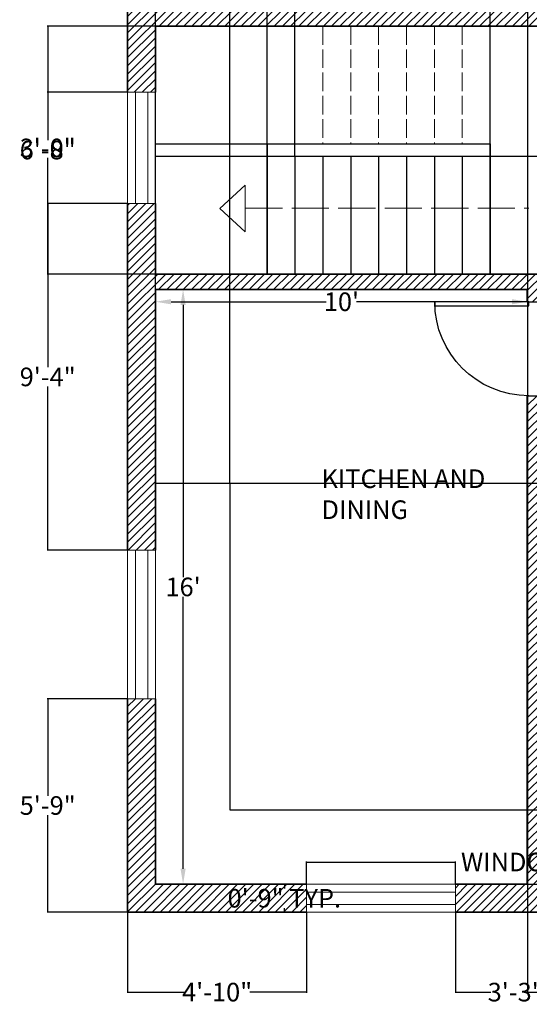
# Model space of a CAD drawing. Units: inches. Extents: x -302 to 383, y -29 to 550.
# Tile 1 of 4: x -17 to 147, y -9 to 308. Entities that reach past the tile are written whole.
import ezdxf

# ---------------------------------------------------------------- set-up
doc = ezdxf.new("R2010")
doc.units = ezdxf.units.IN
doc.header["$MEASUREMENT"] = 0
doc.linetypes.add('ACAD_ISO02W100', pattern=[15, 12, -3])
for name, color, linetype, lineweight in [('A-ANNO-DIMS', 3, 'Continuous', 18), ('A-ANNO-SYMB', 7, 'ACAD_ISO02W100', 18), ('A-AREA-IDEN', 2, 'Continuous', 25), ('A-DOOR', 4, 'Continuous', 25), ('A-FLOR-CASE', 7, 'Continuous', 25), ('A-FLOR-STRS', 7, 'Continuous', 25), ('A-FLOR-STRS-OVHD', 7, 'ACAD_ISO02W100', 18), ('A-GLAZ', 2, 'Continuous', 18), ('A-WALL', 7, 'Continuous', 35), ('A-WALL-PATT', 252, 'Continuous', 13)]:
    doc.layers.add(name, color=color, linetype=linetype, lineweight=lineweight)
doc.styles.get("Standard").update_dxf_attribs({"font": 'arial.ttf'})
doc.dimstyles.get("Standard").update_dxf_attribs({"dimtxt": 6, "dimasz": 0.18, "dimexe": 0.18, "dimexo": 0.0625, "dimgap": 0.09, "dimtad": 0, "dimtih": 1, "dimtoh": 1, "dimzin": 0, "dimdsep": 46, "dimlunit": 3, "dimtxsty": 'Standard', "dimcen": 0.09, "dimadec": 0, "dimazin": 0, "dimtfac": 1, "dimtofl": 0, "dimtmove": 0, "dimatfit": 3, "dimfxl": 1, "dimtolj": 1, "dimtzin": 0, "dimarcsym": 0})

# ---------------------------------------------------------------- blocks, each defined once
blk = doc.blocks.new('*U2')
for p, q in [((0, 0), (0, -6)), ((40, 0), (40, -6))]:
    blk.add_line(p, q)
blk.add_lwpolyline([(0, 0), (0, 40), (1.75, 40), (1.75, 0)], close=True)
blk.add_arc((0, 0), 40, 0, 90)
blk = doc.blocks.new('*D19')
at = {"layer": 'A-ANNO-DIMS', "color": 0, "lineweight": -2, "transparency": 16777216}
for p, q in [((26.76, 221.27), (35.77, 221.27)), ((35.59, 216.27), (35.59, 128.43)), ((35.59, 34.27), (35.59, 122.12)), ((26.76, 29.27), (35.77, 29.27))]:
    blk.add_line(p, q, dxfattribs=at)
at = {"layer": 'A-ANNO-DIMS', "color": 0, "transparency": 16777216}
for points in [[(34.76, 216.27), (36.42, 216.27), (35.59, 221.27)], [(34.76, 34.27), (36.42, 34.27), (35.59, 29.27)]]:
    blk.add_solid(points, dxfattribs=at)
at = {"layer": 'Defpoints', "color": 0, "transparency": 16777216}
for p in [(26.7, 221.27), (26.7, 29.27), (35.59, 29.27)]:
    blk.add_point(p, dxfattribs=at)
at = {"layer": 'A-ANNO-DIMS', "color": 0, "transparency": 16777216, "insert": (35.59, 125.27), "char_height": 6, "attachment_point": 5}
blk.add_mtext("\\A1;16'", dxfattribs=at)
blk = doc.blocks.new('*D20')
at = {"layer": 'A-ANNO-DIMS', "color": 0, "lineweight": -2, "transparency": 16777216}
for p, q in [((26.7, 221.21), (26.7, 217.14)), ((31.7, 217.32), (81.8, 217.32)), ((141.7, 217.32), (91.6, 217.32)), ((146.7, 217.39), (146.7, 217.5))]:
    blk.add_line(p, q, dxfattribs=at)
at = {"layer": 'A-ANNO-DIMS', "color": 0, "transparency": 16777216}
for points in [[(31.7, 218.16), (31.7, 216.49), (26.7, 217.32)], [(141.7, 218.16), (141.7, 216.49), (146.7, 217.32)]]:
    blk.add_solid(points, dxfattribs=at)
at = {"layer": 'Defpoints', "color": 0, "transparency": 16777216}
for p in [(26.7, 221.27), (146.7, 217.32), (146.7, 217.32)]:
    blk.add_point(p, dxfattribs=at)
at = {"layer": 'A-ANNO-DIMS', "color": 0, "transparency": 16777216, "insert": (86.7, 217.32), "char_height": 6, "attachment_point": 5}
blk.add_mtext("\\A1;10'", dxfattribs=at)
blk = doc.blocks.new('WIN-48IN')
blk.add_lwpolyline([(0, 9), (48, 9), (48, 0), (0, 0)], close=True)
for points in [[(0, 6.5), (48, 6.5)], [(0, 2.5), (48, 2.5)]]:
    blk.add_lwpolyline(points)
blk = doc.blocks.new('*D29')
at = {"layer": 'A-ANNO-DIMS', "color": 0, "lineweight": -2, "transparency": 16777216}
for p, q in [((75.47, 29.34), (75.47, 36.65)), ((75.65, 36.47), (123.29, 36.47)), ((123.47, 29.34), (123.47, 36.65)), ((123.47, 36.47), (123.65, 36.47))]:
    blk.add_line(p, q, dxfattribs=at)
at = {"layer": 'A-ANNO-DIMS', "color": 0, "transparency": 16777216}
for points in [[(75.65, 36.5), (75.65, 36.44), (75.47, 36.47)], [(123.29, 36.5), (123.29, 36.44), (123.47, 36.47)]]:
    blk.add_solid(points, dxfattribs=at)
at = {"layer": 'Defpoints', "color": 0, "transparency": 16777216}
for p in [(123.47, 36.47), (75.47, 29.27), (123.47, 29.27)]:
    blk.add_point(p, dxfattribs=at)
at = {"layer": 'A-ANNO-DIMS', "color": 0, "transparency": 16777216, "insert": (161.7, 36.47), "char_height": 6, "attachment_point": 5}
blk.add_mtext('\\A1;WINDOW 4\'-0" TYP.', dxfattribs=at)
blk = doc.blocks.new('*D30')
at = {"layer": 'A-ANNO-DIMS', "color": 0, "lineweight": -2, "transparency": 16777216}
for p, q in [((75.41, 29.27), (68.09, 29.27)), ((68.27, 29.09), (68.27, 27.93)), ((75.41, 20.27), (68.09, 20.27)), ((68.27, 20.45), (68.27, 21.62))]:
    blk.add_line(p, q, dxfattribs=at)
at = {"layer": 'A-ANNO-DIMS', "color": 0, "transparency": 16777216}
for points in [[(68.24, 29.09), (68.3, 29.09), (68.27, 29.27)], [(68.24, 20.45), (68.3, 20.45), (68.27, 20.27)]]:
    blk.add_solid(points, dxfattribs=at)
at = {"layer": 'Defpoints', "color": 0, "transparency": 16777216}
for p in [(68.27, 29.27), (75.47, 29.27), (75.47, 20.27)]:
    blk.add_point(p, dxfattribs=at)
at = {"layer": 'A-ANNO-DIMS', "color": 0, "transparency": 16777216, "insert": (68.27, 24.77), "char_height": 6, "attachment_point": 5}
blk.add_mtext('\\A1;0\'-9" TYP.', dxfattribs=at)
blk = doc.blocks.new('*D37')
at = {"layer": 'A-ANNO-DIMS', "color": 0, "lineweight": -2, "transparency": 16777216}
for p, q in [((17.7, 20.21), (17.7, -5.71)), ((75.47, 20.21), (75.47, -5.71)), ((17.88, -5.53), (36.07, -5.53)), ((75.29, -5.53), (57.1, -5.53))]:
    blk.add_line(p, q, dxfattribs=at)
at = {"layer": 'A-ANNO-DIMS', "color": 0, "transparency": 16777216}
for points in [[(17.88, -5.5), (17.88, -5.56), (17.7, -5.53)], [(75.29, -5.5), (75.29, -5.56), (75.47, -5.53)]]:
    blk.add_solid(points, dxfattribs=at)
at = {"layer": 'Defpoints', "color": 0, "transparency": 16777216}
for p in [(17.7, 20.27), (75.47, 20.27), (75.47, -5.53)]:
    blk.add_point(p, dxfattribs=at)
at = {"layer": 'A-ANNO-DIMS', "color": 0, "transparency": 16777216, "insert": (46.58, -5.53), "char_height": 6, "attachment_point": 5}
blk.add_mtext('\\A1;4\'-10"', dxfattribs=at)
blk = doc.blocks.new('*D38')
at = {"layer": 'A-ANNO-DIMS', "color": 0, "lineweight": -2, "transparency": 16777216}
for p, q in [((123.47, 20.21), (123.47, -5.71)), ((162.44, 20.21), (162.44, -5.71)), ((123.65, -5.53), (134.89, -5.53)), ((162.26, -5.53), (151.02, -5.53))]:
    blk.add_line(p, q, dxfattribs=at)
at = {"layer": 'A-ANNO-DIMS', "color": 0, "transparency": 16777216}
for points in [[(123.65, -5.5), (123.65, -5.56), (123.47, -5.53)], [(162.26, -5.5), (162.26, -5.56), (162.44, -5.53)]]:
    blk.add_solid(points, dxfattribs=at)
at = {"layer": 'Defpoints', "color": 0, "transparency": 16777216}
for p in [(123.47, 20.27), (162.44, 20.27), (162.44, -5.53)]:
    blk.add_point(p, dxfattribs=at)
at = {"layer": 'A-ANNO-DIMS', "color": 0, "transparency": 16777216, "insert": (142.95, -5.53), "char_height": 6, "attachment_point": 5}
blk.add_mtext('\\A1;3\'-3"', dxfattribs=at)
blk = doc.blocks.new('*D41')
at = {"layer": 'A-ANNO-DIMS', "color": 0, "lineweight": -2, "transparency": 16777216}
for p, q in [((17.63, 89.14), (-8.28, 89.14)), ((-8.1, 88.96), (-8.1, 57.86)), ((-8.1, 20.45), (-8.1, 51.55)), ((17.63, 20.27), (-8.28, 20.27))]:
    blk.add_line(p, q, dxfattribs=at)
at = {"layer": 'A-ANNO-DIMS', "color": 0, "transparency": 16777216}
for points in [[(-8.13, 88.96), (-8.07, 88.96), (-8.1, 89.14)], [(-8.13, 20.45), (-8.07, 20.45), (-8.1, 20.27)]]:
    blk.add_solid(points, dxfattribs=at)
at = {"layer": 'Defpoints', "color": 0, "transparency": 16777216}
for p in [(-8.1, 89.14), (17.7, 89.14), (17.7, 20.27)]:
    blk.add_point(p, dxfattribs=at)
at = {"layer": 'A-ANNO-DIMS', "color": 0, "transparency": 16777216, "insert": (-8.1, 54.71), "char_height": 6, "attachment_point": 5}
blk.add_mtext('\\A1;5\'-9"', dxfattribs=at)
blk = doc.blocks.new('*D42')
at = {"layer": 'A-ANNO-DIMS', "color": 0, "lineweight": -2, "transparency": 16777216}
for p, q in [((17.63, 248.98), (-8.28, 248.98)), ((-8.1, 248.8), (-8.1, 196.22)), ((-8.1, 137.32), (-8.1, 189.91)), ((17.63, 137.14), (-8.28, 137.14))]:
    blk.add_line(p, q, dxfattribs=at)
at = {"layer": 'A-ANNO-DIMS', "color": 0, "transparency": 16777216}
for points in [[(-8.13, 248.8), (-8.07, 248.8), (-8.1, 248.98)], [(-8.13, 137.32), (-8.07, 137.32), (-8.1, 137.14)]]:
    blk.add_solid(points, dxfattribs=at)
at = {"layer": 'Defpoints', "color": 0, "transparency": 16777216}
for p in [(-8.1, 248.98), (17.7, 248.98), (17.7, 137.14)]:
    blk.add_point(p, dxfattribs=at)
at = {"layer": 'A-ANNO-DIMS', "color": 0, "transparency": 16777216, "insert": (-8.1, 193.06), "char_height": 6, "attachment_point": 5}
blk.add_mtext('\\A1;9\'-4"', dxfattribs=at)
blk = doc.blocks.new('*D43')
at = {"layer": 'A-ANNO-DIMS', "color": 0, "lineweight": -2, "transparency": 16777216}
for p, q in [((17.63, 284.93), (-8.28, 284.93)), ((-8.1, 284.75), (-8.1, 270.11)), ((-8.1, 249.16), (-8.1, 263.8)), ((17.63, 248.98), (-8.28, 248.98))]:
    blk.add_line(p, q, dxfattribs=at)
at = {"layer": 'A-ANNO-DIMS', "color": 0, "transparency": 16777216}
for points in [[(-8.13, 284.75), (-8.07, 284.75), (-8.1, 284.93)], [(-8.13, 249.16), (-8.07, 249.16), (-8.1, 248.98)]]:
    blk.add_solid(points, dxfattribs=at)
at = {"layer": 'Defpoints', "color": 0, "transparency": 16777216}
for p in [(-8.1, 284.93), (17.7, 284.93), (17.7, 248.98)]:
    blk.add_point(p, dxfattribs=at)
at = {"layer": 'A-ANNO-DIMS', "color": 0, "transparency": 16777216, "insert": (-8.1, 266.96), "char_height": 6, "attachment_point": 5}
blk.add_mtext('\\A1;3\'-0"', dxfattribs=at)
blk = doc.blocks.new('*D51')
at = {"layer": 'A-ANNO-DIMS', "color": 0, "lineweight": -2, "transparency": 16777216}
for p, q in [((146.76, 217.32), (367.68, 217.32)), ((367.5, 217.14), (367.5, 205.35)), ((367.5, 187.18), (367.5, 198.97)), ((146.76, 187), (367.68, 187))]:
    blk.add_line(p, q, dxfattribs=at)
at = {"layer": 'A-ANNO-DIMS', "color": 0, "transparency": 16777216}
for points in [[(367.47, 217.14), (367.53, 217.14), (367.5, 217.32)], [(367.47, 187.18), (367.53, 187.18), (367.5, 187)]]:
    blk.add_solid(points, dxfattribs=at)
at = {"layer": 'Defpoints', "color": 0, "transparency": 16777216}
for p in [(146.7, 217.32), (367.5, 217.32), (146.7, 187)]:
    blk.add_point(p, dxfattribs=at)
at = {"layer": 'A-ANNO-DIMS', "color": 0, "transparency": 16777216, "insert": (367.5, 202.16), "char_height": 6, "attachment_point": 5}
blk.add_mtext('\\A1;2\'-6 1/2"', dxfattribs=at)
blk = doc.blocks.new('*D54')
at = {"layer": 'A-ANNO-DIMS', "color": 0, "lineweight": -2, "transparency": 16777216}
for p, q in [((26.7, 226.34), (26.7, 541.25)), ((26.88, 541.07), (36.63, 541.07)), ((62.52, 541.07), (52.76, 541.07)), ((62.7, 226.34), (62.7, 541.25))]:
    blk.add_line(p, q, dxfattribs=at)
at = {"layer": 'A-ANNO-DIMS', "color": 0, "transparency": 16777216}
for points in [[(26.88, 541.1), (26.88, 541.04), (26.7, 541.07)], [(62.52, 541.1), (62.52, 541.04), (62.7, 541.07)]]:
    blk.add_solid(points, dxfattribs=at)
at = {"layer": 'Defpoints', "color": 0, "transparency": 16777216}
for p in [(62.7, 541.07), (26.7, 226.27), (62.7, 226.27)]:
    blk.add_point(p, dxfattribs=at)
at = {"layer": 'A-ANNO-DIMS', "color": 0, "transparency": 16777216, "insert": (44.7, 541.07), "char_height": 6, "attachment_point": 5}
blk.add_mtext('\\A1;3\'-0"', dxfattribs=at)
blk = doc.blocks.new('*D55')
at = {"layer": 'A-ANNO-DIMS', "color": 0, "lineweight": -2, "transparency": 16777216}
for p, q in [((62.7, 226.34), (62.7, 541.25)), ((62.88, 541.07), (90.62, 541.07)), ((134.52, 541.07), (106.78, 541.07)), ((134.7, 226.34), (134.7, 541.25))]:
    blk.add_line(p, q, dxfattribs=at)
at = {"layer": 'A-ANNO-DIMS', "color": 0, "transparency": 16777216}
for points in [[(62.88, 541.1), (62.88, 541.04), (62.7, 541.07)], [(134.52, 541.1), (134.52, 541.04), (134.7, 541.07)]]:
    blk.add_solid(points, dxfattribs=at)
at = {"layer": 'Defpoints', "color": 0, "transparency": 16777216}
for p in [(134.7, 541.07), (62.7, 226.27), (134.7, 226.27)]:
    blk.add_point(p, dxfattribs=at)
at = {"layer": 'A-ANNO-DIMS', "color": 0, "transparency": 16777216, "insert": (98.7, 541.07), "char_height": 6, "attachment_point": 5}
blk.add_mtext('\\A1;6\'-0"', dxfattribs=at)
blk = doc.blocks.new('*D56')
at = {"layer": 'A-ANNO-DIMS', "color": 0, "lineweight": -2, "transparency": 16777216}
for p, q in [((134.76, 264.27), (367.68, 264.27)), ((367.5, 264.09), (367.5, 248.43)), ((367.5, 226.45), (367.5, 242.12)), ((134.76, 226.27), (367.68, 226.27))]:
    blk.add_line(p, q, dxfattribs=at)
at = {"layer": 'A-ANNO-DIMS', "color": 0, "transparency": 16777216}
for points in [[(367.47, 264.09), (367.53, 264.09), (367.5, 264.27)], [(367.47, 226.45), (367.53, 226.45), (367.5, 226.27)]]:
    blk.add_solid(points, dxfattribs=at)
at = {"layer": 'Defpoints', "color": 0, "transparency": 16777216}
for p in [(134.7, 264.27), (367.5, 264.27), (134.7, 226.27)]:
    blk.add_point(p, dxfattribs=at)
at = {"layer": 'A-ANNO-DIMS', "color": 0, "transparency": 16777216, "insert": (367.5, 245.27), "char_height": 6, "attachment_point": 5}
blk.add_mtext('\\A1;3\'-2"', dxfattribs=at)
blk = doc.blocks.new('*D57')
at = {"layer": 'A-ANNO-DIMS', "color": 0, "lineweight": -2, "transparency": 16777216}
for p, q in [((26.7, 158.79), (26.7, 541.25)), ((26.88, 541.07), (30.58, 541.07)), ((50.52, 541.07), (46.81, 541.07)), ((50.7, 158.79), (50.7, 541.25))]:
    blk.add_line(p, q, dxfattribs=at)
at = {"layer": 'A-ANNO-DIMS', "color": 0, "transparency": 16777216}
for points in [[(26.88, 541.1), (26.88, 541.04), (26.7, 541.07)], [(50.52, 541.1), (50.52, 541.04), (50.7, 541.07)]]:
    blk.add_solid(points, dxfattribs=at)
at = {"layer": 'Defpoints', "color": 0, "transparency": 16777216}
for p in [(50.7, 541.07), (26.7, 158.73), (50.7, 158.73)]:
    blk.add_point(p, dxfattribs=at)
at = {"layer": 'A-ANNO-DIMS', "color": 0, "transparency": 16777216, "insert": (38.7, 541.07), "char_height": 6, "attachment_point": 5}
blk.add_mtext('\\A1;2\'-0"', dxfattribs=at)
blk = doc.blocks.new('*D58')
at = {"layer": 'A-ANNO-DIMS', "color": 0, "lineweight": -2, "transparency": 16777216}
for p, q in [((50.76, 158.73), (367.68, 158.73)), ((367.5, 158.55), (367.5, 109.19)), ((367.5, 53.45), (367.5, 102.81)), ((50.76, 53.27), (367.68, 53.27))]:
    blk.add_line(p, q, dxfattribs=at)
at = {"layer": 'A-ANNO-DIMS', "color": 0, "transparency": 16777216}
for points in [[(367.47, 158.55), (367.53, 158.55), (367.5, 158.73)], [(367.47, 53.45), (367.53, 53.45), (367.5, 53.27)]]:
    blk.add_solid(points, dxfattribs=at)
at = {"layer": 'Defpoints', "color": 0, "transparency": 16777216}
for p in [(50.7, 158.73), (367.5, 158.73), (50.7, 53.27)]:
    blk.add_point(p, dxfattribs=at)
at = {"layer": 'A-ANNO-DIMS', "color": 0, "transparency": 16777216, "insert": (367.5, 106), "char_height": 6, "attachment_point": 5}
blk.add_mtext('\\A1;8\'-9 1/2"', dxfattribs=at)
blk = doc.blocks.new('*D68')
at = {"layer": 'A-ANNO-DIMS', "color": 0, "lineweight": -2, "transparency": 16777216}
for p, q in [((62.7, 268.34), (62.7, 541.25)), ((62.88, 541.07), (71.52, 541.07)), ((71.7, 264.34), (71.7, 541.25)), ((71.7, 541.07), (71.88, 541.07))]:
    blk.add_line(p, q, dxfattribs=at)
at = {"layer": 'A-ANNO-DIMS', "color": 0, "transparency": 16777216}
for points in [[(62.88, 541.1), (62.88, 541.04), (62.7, 541.07)], [(71.52, 541.1), (71.52, 541.04), (71.7, 541.07)]]:
    blk.add_solid(points, dxfattribs=at)
at = {"layer": 'Defpoints', "color": 0, "transparency": 16777216}
for p in [(71.7, 541.07), (62.7, 268.27), (71.7, 264.27)]:
    blk.add_point(p, dxfattribs=at)
at = {"layer": 'A-ANNO-DIMS', "color": 0, "transparency": 16777216, "insert": (79.94, 541.07), "char_height": 6, "attachment_point": 5}
blk.add_mtext('\\A1;0\'-9"', dxfattribs=at)
blk = doc.blocks.new('*D69')
at = {"layer": 'A-ANNO-DIMS', "color": 0, "lineweight": -2, "transparency": 16777216}
for p, q in [((146.76, 53.27), (367.68, 53.27)), ((367.5, 53.09), (367.5, 44.43)), ((367.5, 29.45), (367.5, 38.12)), ((146.76, 29.27), (367.68, 29.27))]:
    blk.add_line(p, q, dxfattribs=at)
at = {"layer": 'A-ANNO-DIMS', "color": 0, "transparency": 16777216}
for points in [[(367.47, 53.09), (367.53, 53.09), (367.5, 53.27)], [(367.47, 29.45), (367.53, 29.45), (367.5, 29.27)]]:
    blk.add_solid(points, dxfattribs=at)
at = {"layer": 'Defpoints', "color": 0, "transparency": 16777216}
for p in [(146.7, 53.27), (367.5, 53.27), (146.7, 29.27)]:
    blk.add_point(p, dxfattribs=at)
at = {"layer": 'A-ANNO-DIMS', "color": 0, "transparency": 16777216, "insert": (367.5, 41.27), "char_height": 6, "attachment_point": 5}
blk.add_mtext('\\A1;2\'-0"', dxfattribs=at)
blk = doc.blocks.new('*D70')
at = {"layer": 'A-ANNO-DIMS', "color": 0, "lineweight": -2, "transparency": 16777216}
for p, q in [((26.63, 306.27), (-8.28, 306.27)), ((-8.1, 306.09), (-8.1, 269.43)), ((-8.1, 226.45), (-8.1, 263.12)), ((26.63, 226.27), (-8.28, 226.27))]:
    blk.add_line(p, q, dxfattribs=at)
at = {"layer": 'A-ANNO-DIMS', "color": 0, "transparency": 16777216}
for points in [[(-8.13, 306.09), (-8.07, 306.09), (-8.1, 306.27)], [(-8.13, 226.45), (-8.07, 226.45), (-8.1, 226.27)]]:
    blk.add_solid(points, dxfattribs=at)
at = {"layer": 'Defpoints', "color": 0, "transparency": 16777216}
for p in [(-8.1, 306.27), (26.7, 306.27), (26.7, 226.27)]:
    blk.add_point(p, dxfattribs=at)
at = {"layer": 'A-ANNO-DIMS', "color": 0, "transparency": 16777216, "insert": (-8.1, 266.27), "char_height": 6, "attachment_point": 5}
blk.add_mtext('\\A1;6\'-8"', dxfattribs=at)
blk = doc.blocks.new('*D71')
at = {"layer": 'A-ANNO-DIMS', "color": 0, "lineweight": -2, "transparency": 16777216}
for p, q in [((146.7, 358.81), (146.7, -5.71)), ((151.7, 354.21), (151.7, -5.71)), ((146.88, -5.53), (151.52, -5.53)), ((151.7, -5.53), (151.88, -5.53))]:
    blk.add_line(p, q, dxfattribs=at)
at = {"layer": 'A-ANNO-DIMS', "color": 0, "transparency": 16777216}
for points in [[(146.88, -5.5), (146.88, -5.56), (146.7, -5.53)], [(151.52, -5.5), (151.52, -5.56), (151.7, -5.53)]]:
    blk.add_solid(points, dxfattribs=at)
at = {"layer": 'Defpoints', "color": 0, "transparency": 16777216}
for p in [(146.7, 358.87), (151.7, 354.27), (151.7, -5.53)]:
    blk.add_point(p, dxfattribs=at)
at = {"layer": 'A-ANNO-DIMS', "color": 0, "transparency": 16777216, "insert": (159.94, -5.53), "char_height": 6, "attachment_point": 5}
blk.add_mtext('\\A1;0\'-5"', dxfattribs=at)

msp = doc.modelspace()

# ---------------------------------------------------------------- hatches: boundary and pattern name
at = {"layer": 'A-WALL-PATT'}
h = msp.add_hatch(dxfattribs=at)
h.set_pattern_fill('ANSI31', color=256, scale=15)
h.paths.add_polyline_path([(201.697, 29.273), (187.202, 29.273), (187.202, 20.273), (251.158, 20.273), (251.158, 29.273), (206.697, 29.273), (206.697, 149.273), (294.846, 149.273, -0.0045588), (294.841, 149.815), (294.841, 154.273), (201.697, 154.273), (201.697, 130.273), (190.923, 130.273), (190.923, 125.273), (201.697, 125.273)])
h.paths.add_polyline_path([(341.697, 154.273), (332.697, 154.273), (324.561, 154.273), (324.561, 149.815), (324.561, 149.273), (332.697, 149.273), (332.697, 29.273), (299.158, 29.273), (299.158, 20.273), (341.697, 20.273)])
h.paths.add_polyline_path([(75.47, 20.273), (75.47, 29.273), (26.697, 29.273), (26.697, 89.142), (17.697, 89.142), (17.697, 20.273)])
h.paths.add_polyline_path([(26.697, 221.273), (146.697, 221.273), (146.697, 217.323), (147.147, 217.323), (151.697, 217.323), (151.697, 226.273), (26.697, 226.273), (26.697, 248.984), (17.697, 248.984), (17.697, 137.142), (26.697, 137.142)])
h.paths.add_polyline_path([(17.697, 284.934), (26.697, 284.934), (26.697, 306.273), (151.697, 306.273), (151.697, 317.511), (147.338, 317.511), (146.697, 317.511), (146.697, 311.273), (26.697, 311.273), (26.697, 377.22), (17.697, 377.22)])
h.paths.add_polyline_path([(341.697, 376.674), (332.697, 376.674), (332.697, 311.273), (212.697, 311.273), (212.697, 317.511), (212.055, 317.511), (207.697, 317.511), (207.697, 306.273), (332.697, 306.273), (332.697, 214.273), (341.697, 214.273)])
h.paths.add_polyline_path([(207.697, 455.273), (207.697, 359.273), (202.395, 359.273), (202.395, 357.888), (202.395, 354.273), (207.697, 354.273), (207.697, 346.57), (212.055, 346.57, -0.0055163), (212.697, 346.563), (212.697, 455.273), (332.697, 455.273), (332.697, 424.674), (341.697, 424.674), (341.697, 464.273), (188.075, 464.273), (188.075, 455.273)])
h.paths.add_polyline_path([(17.697, 464.273), (17.697, 425.22), (26.697, 425.22), (26.697, 455.273), (146.697, 455.273), (146.697, 346.563, -0.0055163), (147.338, 346.57), (151.697, 346.57), (151.697, 354.273), (178.3, 354.273), (178.3, 357.888, -0.0143868), (178.34, 359.273), (151.697, 359.273), (151.697, 455.273), (162.634, 455.273), (162.634, 464.273)])
h = msp.add_hatch(dxfattribs=at)
h.set_pattern_fill('ANSI31', color=256, scale=15)
h.paths.add_polyline_path([(151.697, 186.995), (147.147, 186.995, -0.0037161), (146.697, 186.998), (146.697, 29.273), (123.47, 29.273), (123.47, 20.273), (162.437, 20.273), (162.437, 29.273), (151.697, 29.273), (151.697, 125.273), (157.23, 125.273), (157.23, 130.273), (151.697, 130.273)])

# ---------------------------------------------------------------- linework, layer by layer
at = {"layer": 'A-ANNO-SYMB'}
msp.add_line((55.668, 247.478), (147.134, 247.478), dxfattribs=at)
msp.add_lwpolyline([(47.42, 247.402), (55.668, 239.912), (47.42, 247.402), (55.668, 254.974), (55.668, 247.478), (55.668, 239.912)], dxfattribs=at)
at = {"layer": 'A-FLOR-CASE'}
msp.add_line((26.697, 158.726), (50.697, 158.726), dxfattribs=at)
for points in [[(50.697, 158.726), (50.697, 53.273)], [(50.697, 158.726), (50.697, 137.142)], [(50.697, 53.273), (146.697, 53.273)]]:
    msp.add_lwpolyline(points, dxfattribs=at)
at = {"layer": 'A-FLOR-STRS'}
for p, q in [((26.697, 268.273), (134.697, 268.273)), ((26.697, 264.273), (134.697, 264.273))]:
    msp.add_line(p, q, dxfattribs=at)
for points in [[(62.697, 268.273), (62.697, 226.273)], [(134.697, 268.273), (134.697, 226.273)], [(71.697, 264.273), (71.697, 226.273)], [(80.697, 264.273), (80.697, 226.273)], [(89.697, 264.273), (89.697, 226.273)], [(98.697, 264.273), (98.697, 226.273)], [(107.697, 264.273), (107.697, 226.273)], [(116.697, 264.273), (116.697, 226.273)], [(125.697, 264.273), (125.697, 226.273)]]:
    msp.add_lwpolyline(points, dxfattribs=at)
at = {"layer": 'A-FLOR-STRS-OVHD', "ltscale": 0.5}
for points in [[(62.697, 306.273), (62.697, 268.273)], [(71.697, 306.273), (71.697, 268.273)], [(80.697, 306.273), (80.697, 268.273)], [(89.697, 306.273), (89.697, 268.273)], [(98.697, 306.273), (98.697, 268.273)], [(107.697, 306.273), (107.697, 268.273)], [(116.697, 306.273), (116.697, 268.273)], [(125.697, 306.273), (125.697, 268.273)], [(134.697, 306.273), (134.697, 268.273)]]:
    msp.add_lwpolyline(points, dxfattribs=at)
at = {"layer": 'A-GLAZ'}
msp.add_lwpolyline([(17.697, 284.934), (26.697, 284.934), (26.697, 248.984), (17.697, 248.984)], close=True, dxfattribs=at)
for points in [[(20.197, 284.934), (20.197, 248.984)], [(24.197, 284.934), (24.197, 248.984)]]:
    msp.add_lwpolyline(points, dxfattribs=at)
at = {"layer": 'A-WALL'}
for points in [[(17.697, 377.22), (17.697, 284.934)], [(151.697, 306.273), (26.697, 306.273)], [(26.697, 306.273), (26.697, 284.934)], [(17.697, 248.984), (17.697, 137.142)], [(26.697, 248.984), (26.697, 226.273)], [(26.697, 226.273), (151.697, 226.273)], [(26.697, 221.273), (146.697, 221.273)], [(26.697, 221.273), (26.697, 137.142)], [(146.697, 221.273), (146.697, 217.323)], [(146.697, 186.998), (146.697, 29.273)], [(17.697, 89.142), (17.697, 20.273), (75.47, 20.273)], [(26.697, 89.142), (26.697, 29.273)], [(26.697, 29.273), (75.47, 29.273)], [(123.47, 29.273), (146.697, 29.273)], [(123.47, 20.273), (162.437, 20.273)]]:
    msp.add_lwpolyline(points, dxfattribs=at)

# ---------------------------------------------------------------- block references
at = {"layer": 'A-DOOR', "xscale": -0.7582020296560713, "yscale": 0.7582020296560713, "zscale": 0.7582020296560713, "rotation": 90}
msp.add_blockref('*U2', (147.147, 217.323), dxfattribs=at)
at = {"layer": 'A-GLAZ', "extrusion": (0, 0, -1), "zscale": -1, "rotation": 270}
msp.add_blockref('WIN-48IN', (-26.697, 137.142), dxfattribs=at)
at = {"layer": 'A-GLAZ'}
msp.add_blockref('WIN-48IN', (75.47, 20.273), dxfattribs=at)

# ---------------------------------------------------------------- texts
at = {"layer": 'A-AREA-IDEN', "insert": (80.282, 163.197), "char_height": 6, "attachment_point": 1}
msp.add_mtext_dynamic_manual_height_columns('{KITCHEN AND  DINING}', width=74.36308, gutter_width=1, heights=[0], dxfattribs=at)

# ---------------------------------------------------------------- dimensions: what is measured, and where the dimension line sits
at = {"layer": 'A-ANNO-DIMS'}
for base, p1, p2, override, picture, middle in [((62.697, 541.073), (26.697, 226.273), (62.697, 226.273), {"dimdec": 1, "dimlfac": 1, "dimrnd": 0, "dimzin": 1, "dimdsep": 46, "dimlunit": 4, "dimfrac": 2}, '*D54', (44.697, 541.073)), ((50.697, 541.073), (26.697, 158.726), (50.697, 158.726), {"dimdec": 1, "dimlfac": 1, "dimrnd": 0, "dimzin": 1, "dimdsep": 46, "dimlunit": 4, "dimfrac": 2}, '*D57', (38.697, 541.073)), ((134.697, 541.073), (62.697, 226.273), (134.697, 226.273), {"dimdec": 1, "dimlfac": 1, "dimrnd": 0, "dimzin": 1, "dimdsep": 46, "dimlunit": 4, "dimfrac": 2}, '*D55', (98.697, 541.073)), ((71.697, 541.073), (62.697, 268.273), (71.697, 264.273), {"dimdec": 1, "dimlfac": 1, "dimrnd": 0, "dimzin": 1, "dimdsep": 46, "dimlunit": 4, "dimfrac": 2}, '*D68', (79.941, 541.073)), ((151.697, -5.527), (146.697, 358.869), (151.697, 354.273), {"dimdec": 1, "dimlfac": 1, "dimrnd": 0, "dimzin": 1, "dimdsep": 46, "dimlunit": 4, "dimfrac": 2}, '*D71', (159.941, -5.527)), ((146.697, 217.323), (26.697, 221.273), (146.697, 217.323), {"dimasz": 5, "dimclrd": 0, "dimclre": 0, "dimclrt": 0}, '*D20', (86.697, 217.323)), ((75.47, -5.527), (17.697, 20.273), (75.47, 20.273), {"dimdec": 1, "dimlfac": 1, "dimrnd": 0, "dimzin": 1, "dimdsep": 46, "dimlunit": 4, "dimfrac": 2}, '*D37', (46.583, -5.527)), ((162.437, -5.527), (123.47, 20.273), (162.437, 20.273), {"dimdec": 1, "dimlfac": 1, "dimrnd": 0, "dimzin": 1, "dimdsep": 46, "dimlunit": 4, "dimfrac": 2}, '*D38', (142.954, -5.527))]:
    dim = msp.add_linear_dim(base=base, p1=p1, p2=p2, dimstyle='Standard', override=override, dxfattribs=at)
    dim.commit()
    dim.dimension.update_dxf_attribs({"geometry": picture, "text_midpoint": middle})
for base, p1, p2, override, picture, middle in [((-8.103, 306.273), (26.697, 226.273), (26.697, 306.273), {"dimdec": 1, "dimlfac": 1, "dimrnd": 0, "dimzin": 1, "dimdsep": 46, "dimlunit": 4, "dimfrac": 2}, '*D70', (-8.103, 266.273)), ((-8.1034, 284.9339), (17.6966, 248.9836), (17.6966, 284.9339), {"dimdec": 1, "dimlfac": 1, "dimrnd": 0, "dimzin": 1, "dimdsep": 46, "dimlunit": 4, "dimfrac": 2}, '*D43', (-8.1034, 266.9587)), ((367.497, 264.273), (134.697, 226.273), (134.697, 264.273), {"dimdec": 1, "dimlfac": 1, "dimrnd": 0, "dimzin": 1, "dimdsep": 46, "dimlunit": 4, "dimfrac": 2}, '*D56', (367.497, 245.273)), ((-8.103, 248.984), (17.697, 137.142), (17.697, 248.984), {"dimdec": 1, "dimlfac": 1, "dimrnd": 0, "dimzin": 1, "dimdsep": 46, "dimlunit": 4, "dimfrac": 2}, '*D42', (-8.103, 193.063)), ((35.591, 29.273), (26.697, 221.273), (26.697, 29.273), {"dimasz": 5, "dimclrd": 0, "dimclre": 0, "dimclrt": 0}, '*D19', (35.591, 125.273)), ((367.497, 217.323), (146.697, 186.998), (146.697, 217.323), {"dimdec": 1, "dimlfac": 1, "dimrnd": 0, "dimzin": 1, "dimdsep": 46, "dimlunit": 4, "dimfrac": 2}, '*D51', (367.497, 202.16)), ((367.497, 158.726), (50.697, 53.273), (50.697, 158.726), {"dimdec": 1, "dimlfac": 1, "dimrnd": 0, "dimzin": 1, "dimdsep": 46, "dimlunit": 4, "dimfrac": 2}, '*D58', (367.497, 106)), ((-8.103, 89.142), (17.697, 20.273), (17.697, 89.142), {"dimdec": 1, "dimlfac": 1, "dimrnd": 0, "dimzin": 1, "dimdsep": 46, "dimlunit": 4, "dimfrac": 2}, '*D41', (-8.103, 54.708)), ((367.497, 53.273), (146.697, 29.273), (146.697, 53.273), {"dimdec": 1, "dimlfac": 1, "dimrnd": 0, "dimzin": 1, "dimdsep": 46, "dimlunit": 4, "dimfrac": 2}, '*D69', (367.497, 41.273))]:
    dim = msp.add_linear_dim(base=base, p1=p1, p2=p2, angle=90, dimstyle='Standard', override=override, dxfattribs=at)
    dim.commit()
    dim.dimension.update_dxf_attribs({"geometry": picture, "text_midpoint": middle})
dim = msp.add_linear_dim(base=(123.47, 36.473), p1=(75.47, 29.273), p2=(123.47, 29.273), text='WINDOW <> TYP.', dimstyle='Standard', override={"dimdec": 1, "dimlfac": 1, "dimrnd": 0, "dimzin": 1, "dimdsep": 46, "dimlunit": 4, "dimfrac": 2}, dxfattribs=at)
dim.commit()
dim.dimension.update_dxf_attribs({"geometry": '*D29', "text_midpoint": (161.703, 36.473)})
dim = msp.add_linear_dim(base=(68.27, 29.273), p1=(75.47, 20.273), p2=(75.47, 29.273), angle=90, text='<> TYP.', dimstyle='Standard', override={"dimdec": 1, "dimlfac": 1, "dimrnd": 0, "dimzin": 1, "dimdsep": 46, "dimlunit": 4, "dimfrac": 2}, dxfattribs=at)
dim.commit()
dim.dimension.update_dxf_attribs({"geometry": '*D30', "text_midpoint": (68.27, 24.773)})

doc.saveas('drawing.dxf')
